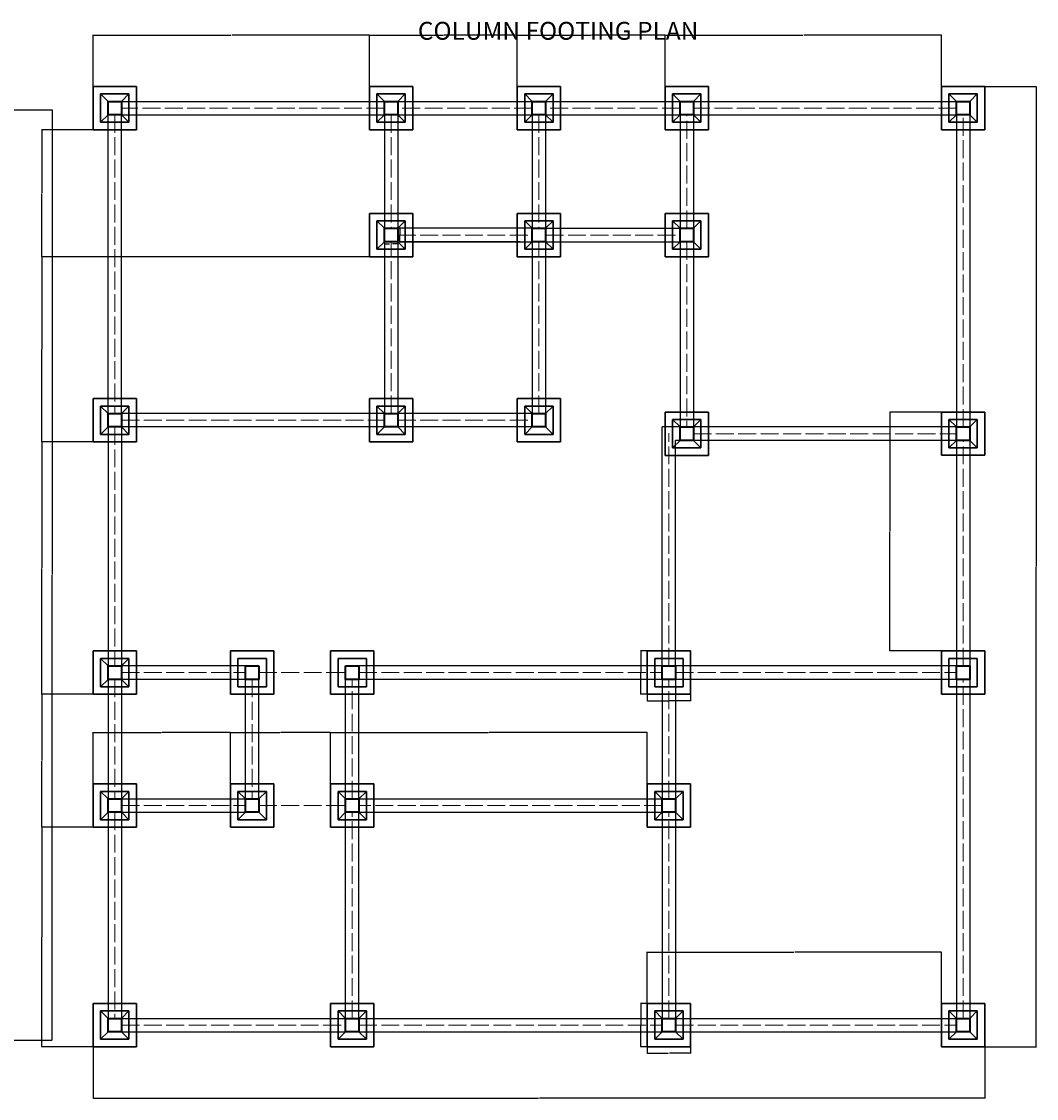
# Model space of a CAD drawing. Units: inches. Extents: x -1138 to 192, y 31 to 760.
# Tile 6 of 6: x -488 to 192, y 39 to 760. Entities that reach past the tile are written whole.
import ezdxf

# ---------------------------------------------------------------- set-up
doc = ezdxf.new("R2010")
doc.units = ezdxf.units.IN
doc.header["$MEASUREMENT"] = 0
doc.linetypes.add('ACAD_ISO02W100', pattern=[15, 12, -3])
for name, color, linetype, lineweight in [('A-ANNO-DIMS', 2, 'Continuous', 18), ('S-ANNO-TEXT', 7, 'Continuous', 25), ('S-BEAM', 7, 'Continuous', 25), ('S-BEAM-CNTR', 3, 'ACAD_ISO02W100', 13), ('S-COLS', 1, 'Continuous', 35), ('S-FNDN', 7, 'Continuous', 30)]:
    doc.layers.add(name, color=color, linetype=linetype, lineweight=lineweight)
doc.styles.get("Standard").update_dxf_attribs({"font": 'arial.ttf'})
doc.dimstyles.get("Standard").update_dxf_attribs({"dimtxt": 0.18, "dimasz": 0.18, "dimexe": 0.18, "dimexo": 0.0625, "dimgap": 0.09, "dimtad": 0, "dimtih": 1, "dimtoh": 1, "dimdec": 1, "dimzin": 0, "dimdsep": 46, "dimlunit": 4, "dimtxsty": 'Standard', "dimcen": 0.09, "dimadec": 0, "dimazin": 0, "dimtfac": 1, "dimtdec": 1, "dimtofl": 0, "dimtmove": 0, "dimatfit": 3, "dimfxl": 1, "dimtolj": 1, "dimtzin": 0, "dimarcsym": 0})

# ---------------------------------------------------------------- blocks, each defined once
blk = doc.blocks.new('COL-SQUARE-9IN')
for p, q in [((0, 9), (9, 9)), ((0, 0), (0, 9)), ((9, 9), (9, 0)), ((9, 0), (0, 0))]:
    blk.add_line(p, q)
blk = doc.blocks.new('FTG-29IN-SLOPED')
for p, q in [((0, 0), (0, 29)), ((0, 29), (29, 29)), ((29, 29), (29, 0)), ((5, 5), (5, 24)), ((5, 24), (24, 24)), ((5, 24), (10, 19)), ((19, 19), (24, 24)), ((24, 24), (24, 5)), ((5, 5), (10, 10)), ((19, 10), (24, 5)), ((24, 5), (5, 5)), ((29, 0), (0, 0))]:
    blk.add_line(p, q)
blk = doc.blocks.new('FTG-29IN-STEPPED')
for p, q in [((0, 0), (0, 29)), ((0, 29), (29, 29)), ((29, 29), (29, 0)), ((5, 5), (5, 24)), ((5, 24), (24, 24)), ((24, 24), (24, 5)), ((24, 5), (5, 5)), ((29, 0), (0, 0))]:
    blk.add_line(p, q)
blk = doc.blocks.new('*D39')
at = {"layer": 'A-ANNO-DIMS', "color": 0, "lineweight": -2, "transparency": 16777216}
for p, q in [((-244.81, 612.31), (-244.81, 610.84)), ((-244.63, 611.02), (-241.35, 611.02)), ((-235.99, 611.02), (-239.27, 611.02)), ((-235.81, 612.31), (-235.81, 610.84))]:
    blk.add_line(p, q, dxfattribs=at)
at = {"layer": 'A-ANNO-DIMS', "color": 0, "transparency": 16777216}
for points in [[(-244.63, 611.05), (-244.63, 610.99), (-244.81, 611.02)], [(-235.99, 611.05), (-235.99, 610.99), (-235.81, 611.02)]]:
    blk.add_solid(points, dxfattribs=at)
at = {"layer": 'Defpoints', "color": 0, "transparency": 16777216}
for p in [(-244.81, 612.37), (-235.81, 612.37), (-235.81, 611.02)]:
    blk.add_point(p, dxfattribs=at)
at = {"layer": 'A-ANNO-DIMS', "color": 0, "transparency": 16777216, "insert": (-240.31, 611.02), "char_height": 0.18, "attachment_point": 5}
blk.add_mtext('\\A1;COLUMN 9 TYP.', dxfattribs=at)
blk = doc.blocks.new('*D40')
at = {"layer": 'A-ANNO-DIMS', "color": 0, "lineweight": -2, "transparency": 16777216}
for p, q in [((-235.75, 621.37), (-234.28, 621.37)), ((-234.46, 621.19), (-234.46, 617.05)), ((-234.46, 612.55), (-234.46, 616.69)), ((-235.75, 612.37), (-234.28, 612.37))]:
    blk.add_line(p, q, dxfattribs=at)
at = {"layer": 'A-ANNO-DIMS', "color": 0, "transparency": 16777216}
for points in [[(-234.49, 621.19), (-234.43, 621.19), (-234.46, 621.37)], [(-234.49, 612.55), (-234.43, 612.55), (-234.46, 612.37)]]:
    blk.add_solid(points, dxfattribs=at)
at = {"layer": 'Defpoints', "color": 0, "transparency": 16777216}
for p in [(-235.81, 621.37), (-234.46, 621.37), (-235.81, 612.37)]:
    blk.add_point(p, dxfattribs=at)
at = {"layer": 'A-ANNO-DIMS', "color": 0, "transparency": 16777216, "insert": (-234.46, 616.87), "char_height": 0.18, "attachment_point": 5}
blk.add_mtext('\\A1;9 TYP.', dxfattribs=at)
blk = doc.blocks.new('*D41')
at = {"layer": 'A-ANNO-DIMS', "color": 0, "lineweight": -2, "transparency": 16777216}
for p, q in [((-68.87, 102.37), (-73.34, 102.37)), ((-73.16, 102.19), (-73.16, 88.05)), ((-73.16, 73.55), (-73.16, 87.69)), ((-68.87, 73.37), (-73.34, 73.37))]:
    blk.add_line(p, q, dxfattribs=at)
at = {"layer": 'A-ANNO-DIMS', "color": 0, "transparency": 16777216}
for points in [[(-73.19, 102.19), (-73.13, 102.19), (-73.16, 102.37)], [(-73.19, 73.55), (-73.13, 73.55), (-73.16, 73.37)]]:
    blk.add_solid(points, dxfattribs=at)
at = {"layer": 'Defpoints', "color": 0, "transparency": 16777216}
for p in [(-68.81, 102.37), (-73.16, 73.37), (-68.81, 73.37)]:
    blk.add_point(p, dxfattribs=at)
at = {"layer": 'A-ANNO-DIMS', "color": 0, "transparency": 16777216, "insert": (-73.16, 87.87), "char_height": 0.18, "attachment_point": 5}
blk.add_mtext('\\A1;SLOPED FOOTING 29 TYP.', dxfattribs=at)
blk = doc.blocks.new('*D42')
at = {"layer": 'A-ANNO-DIMS', "color": 0, "lineweight": -2, "transparency": 16777216}
for p, q in [((-68.81, 73.31), (-68.81, 68.84)), ((-39.81, 73.31), (-39.81, 68.84)), ((-68.63, 69.02), (-54.84, 69.02)), ((-39.99, 69.02), (-53.78, 69.02))]:
    blk.add_line(p, q, dxfattribs=at)
at = {"layer": 'A-ANNO-DIMS', "color": 0, "transparency": 16777216}
for points in [[(-68.63, 69.05), (-68.63, 68.99), (-68.81, 69.02)], [(-39.99, 69.05), (-39.99, 68.99), (-39.81, 69.02)]]:
    blk.add_solid(points, dxfattribs=at)
at = {"layer": 'Defpoints', "color": 0, "transparency": 16777216}
for p in [(-68.81, 73.37), (-39.81, 73.37), (-39.81, 69.02)]:
    blk.add_point(p, dxfattribs=at)
at = {"layer": 'A-ANNO-DIMS', "color": 0, "transparency": 16777216, "insert": (-54.31, 69.02), "char_height": 0.18, "attachment_point": 5}
blk.add_mtext('\\A1;29 TYP.', dxfattribs=at)
blk = doc.blocks.new('*D43')
at = {"layer": 'A-ANNO-DIMS', "color": 0, "lineweight": -2, "transparency": 16777216}
for p, q in [((-68.87, 338.37), (-73.34, 338.37)), ((-73.16, 338.19), (-73.16, 324.05)), ((-73.16, 309.55), (-73.16, 323.69)), ((-68.87, 309.37), (-73.34, 309.37))]:
    blk.add_line(p, q, dxfattribs=at)
at = {"layer": 'A-ANNO-DIMS', "color": 0, "transparency": 16777216}
for points in [[(-73.19, 338.19), (-73.13, 338.19), (-73.16, 338.37)], [(-73.19, 309.55), (-73.13, 309.55), (-73.16, 309.37)]]:
    blk.add_solid(points, dxfattribs=at)
at = {"layer": 'Defpoints', "color": 0, "transparency": 16777216}
for p in [(-68.81, 338.37), (-73.16, 309.37), (-68.81, 309.37)]:
    blk.add_point(p, dxfattribs=at)
at = {"layer": 'A-ANNO-DIMS', "color": 0, "transparency": 16777216, "insert": (-73.16, 323.87), "char_height": 0.18, "attachment_point": 5}
blk.add_mtext('\\A1;STEPPED FOOTING 29 TYP.', dxfattribs=at)
blk = doc.blocks.new('*D44')
at = {"layer": 'A-ANNO-DIMS', "color": 0, "lineweight": -2, "transparency": 16777216}
for p, q in [((-68.81, 309.31), (-68.81, 304.84)), ((-68.63, 305.02), (-54.84, 305.02)), ((-39.99, 305.02), (-53.78, 305.02)), ((-39.81, 309.31), (-39.81, 304.84))]:
    blk.add_line(p, q, dxfattribs=at)
at = {"layer": 'A-ANNO-DIMS', "color": 0, "transparency": 16777216}
for points in [[(-68.63, 305.05), (-68.63, 304.99), (-68.81, 305.02)], [(-39.99, 305.05), (-39.99, 304.99), (-39.81, 305.02)]]:
    blk.add_solid(points, dxfattribs=at)
at = {"layer": 'Defpoints', "color": 0, "transparency": 16777216}
for p in [(-68.81, 309.37), (-39.81, 309.37), (-39.81, 305.02)]:
    blk.add_point(p, dxfattribs=at)
at = {"layer": 'A-ANNO-DIMS', "color": 0, "transparency": 16777216, "insert": (-54.31, 305.02), "char_height": 0.18, "attachment_point": 5}
blk.add_mtext('\\A1;29 TYP.', dxfattribs=at)
blk = doc.blocks.new('*D86')
at = {"layer": 'A-ANNO-DIMS', "color": 0, "lineweight": -2, "transparency": 16777216}
for p, q in [((-514.07, 700.81), (-467.14, 700.81)), ((-467.32, 700.63), (-467.32, 389.49)), ((-467.32, 77.99), (-467.32, 389.13)), ((-514.07, 77.81), (-467.14, 77.81))]:
    blk.add_line(p, q, dxfattribs=at)
at = {"layer": 'A-ANNO-DIMS', "color": 0, "transparency": 16777216}
for points in [[(-467.35, 700.63), (-467.29, 700.63), (-467.32, 700.81)], [(-467.35, 77.99), (-467.29, 77.99), (-467.32, 77.81)]]:
    blk.add_solid(points, dxfattribs=at)
at = {"layer": 'Defpoints', "color": 0, "transparency": 16777216}
for p in [(-514.13, 700.81), (-467.32, 700.81), (-514.13, 77.81)]:
    blk.add_point(p, dxfattribs=at)
at = {"layer": 'A-ANNO-DIMS', "color": 0, "transparency": 16777216, "insert": (-467.32, 389.31), "char_height": 0.18, "attachment_point": 5}
blk.add_mtext('\\A1;623', dxfattribs=at)
blk = doc.blocks.new('*D105')
at = {"layer": 'A-ANNO-DIMS', "color": 0, "lineweight": -2, "transparency": 16777216}
for p, q in [((-439.81, 73.31), (-439.81, 38.76)), ((157.19, 73.31), (157.19, 38.76)), ((-439.63, 38.94), (-141.6, 38.94)), ((157.01, 38.94), (-141.02, 38.94))]:
    blk.add_line(p, q, dxfattribs=at)
at = {"layer": 'A-ANNO-DIMS', "color": 0, "transparency": 16777216}
for points in [[(-439.63, 38.97), (-439.63, 38.91), (-439.81, 38.94)], [(157.01, 38.97), (157.01, 38.91), (157.19, 38.94)]]:
    blk.add_solid(points, dxfattribs=at)
at = {"layer": 'Defpoints', "color": 0, "transparency": 16777216}
for p in [(-439.81, 73.37), (157.19, 73.37), (157.19, 38.94)]:
    blk.add_point(p, dxfattribs=at)
at = {"layer": 'A-ANNO-DIMS', "color": 0, "transparency": 16777216, "insert": (-141.31, 38.94), "char_height": 0.18, "attachment_point": 5}
blk.add_mtext('\\A1;597', dxfattribs=at)
blk = doc.blocks.new('*D106')
at = {"layer": 'A-ANNO-DIMS', "color": 0, "lineweight": -2, "transparency": 16777216}
for p, q in [((157.25, 716.37), (191.81, 716.37)), ((191.63, 716.19), (191.63, 395.05)), ((191.63, 73.55), (191.63, 394.69)), ((157.25, 73.37), (191.81, 73.37))]:
    blk.add_line(p, q, dxfattribs=at)
at = {"layer": 'A-ANNO-DIMS', "color": 0, "transparency": 16777216}
for points in [[(191.6, 716.19), (191.66, 716.19), (191.63, 716.37)], [(191.6, 73.55), (191.66, 73.55), (191.63, 73.37)]]:
    blk.add_solid(points, dxfattribs=at)
at = {"layer": 'Defpoints', "color": 0, "transparency": 16777216}
for p in [(157.19, 716.37), (191.63, 716.37), (157.19, 73.37)]:
    blk.add_point(p, dxfattribs=at)
at = {"layer": 'A-ANNO-DIMS', "color": 0, "transparency": 16777216, "insert": (191.63, 394.87), "char_height": 0.18, "attachment_point": 5}
blk.add_mtext('\\A1;643', dxfattribs=at)
blk = doc.blocks.new('*D107')
at = {"layer": 'A-ANNO-DIMS', "color": 0, "lineweight": -2, "transparency": 16777216}
for p, q in [((-439.81, 716.43), (-439.81, 750.99)), ((-439.63, 750.81), (-347.59, 750.81)), ((-254.99, 750.81), (-347.03, 750.81)), ((-254.81, 716.43), (-254.81, 750.99))]:
    blk.add_line(p, q, dxfattribs=at)
at = {"layer": 'A-ANNO-DIMS', "color": 0, "transparency": 16777216}
for points in [[(-439.63, 750.84), (-439.63, 750.78), (-439.81, 750.81)], [(-254.99, 750.84), (-254.99, 750.78), (-254.81, 750.81)]]:
    blk.add_solid(points, dxfattribs=at)
at = {"layer": 'Defpoints', "color": 0, "transparency": 16777216}
for p in [(-254.81, 750.81), (-439.81, 716.37), (-254.81, 716.37)]:
    blk.add_point(p, dxfattribs=at)
at = {"layer": 'A-ANNO-DIMS', "color": 0, "transparency": 16777216, "insert": (-347.31, 750.81), "char_height": 0.18, "attachment_point": 5}
blk.add_mtext('\\A1;185', dxfattribs=at)
blk = doc.blocks.new('*D108')
at = {"layer": 'A-ANNO-DIMS', "color": 0, "lineweight": -2, "transparency": 16777216}
for p, q in [((-254.81, 716.43), (-254.81, 750.99)), ((-254.63, 750.81), (-205.53, 750.81)), ((-155.99, 750.81), (-205.09, 750.81)), ((-155.81, 716.43), (-155.81, 750.99))]:
    blk.add_line(p, q, dxfattribs=at)
at = {"layer": 'A-ANNO-DIMS', "color": 0, "transparency": 16777216}
for points in [[(-254.63, 750.84), (-254.63, 750.78), (-254.81, 750.81)], [(-155.99, 750.84), (-155.99, 750.78), (-155.81, 750.81)]]:
    blk.add_solid(points, dxfattribs=at)
at = {"layer": 'Defpoints', "color": 0, "transparency": 16777216}
for p in [(-155.81, 750.81), (-254.81, 716.37), (-155.81, 716.37)]:
    blk.add_point(p, dxfattribs=at)
at = {"layer": 'A-ANNO-DIMS', "color": 0, "transparency": 16777216, "insert": (-205.31, 750.81), "char_height": 0.18, "attachment_point": 5}
blk.add_mtext('\\A1;99', dxfattribs=at)
blk = doc.blocks.new('*D109')
at = {"layer": 'A-ANNO-DIMS', "color": 0, "lineweight": -2, "transparency": 16777216}
for p, q in [((-155.81, 716.43), (-155.81, 750.99)), ((-155.63, 750.81), (-106.53, 750.81)), ((-56.99, 750.81), (-106.09, 750.81)), ((-56.81, 716.43), (-56.81, 750.99))]:
    blk.add_line(p, q, dxfattribs=at)
at = {"layer": 'A-ANNO-DIMS', "color": 0, "transparency": 16777216}
for points in [[(-155.63, 750.84), (-155.63, 750.78), (-155.81, 750.81)], [(-56.99, 750.84), (-56.99, 750.78), (-56.81, 750.81)]]:
    blk.add_solid(points, dxfattribs=at)
at = {"layer": 'Defpoints', "color": 0, "transparency": 16777216}
for p in [(-56.81, 750.81), (-155.81, 716.37), (-56.81, 716.37)]:
    blk.add_point(p, dxfattribs=at)
at = {"layer": 'A-ANNO-DIMS', "color": 0, "transparency": 16777216, "insert": (-106.31, 750.81), "char_height": 0.18, "attachment_point": 5}
blk.add_mtext('\\A1;99', dxfattribs=at)
blk = doc.blocks.new('*D110')
at = {"layer": 'A-ANNO-DIMS', "color": 0, "lineweight": -2, "transparency": 16777216}
for p, q in [((-56.81, 716.43), (-56.81, 750.99)), ((-56.63, 750.81), (35.41, 750.81)), ((128.01, 750.81), (35.97, 750.81)), ((128.19, 716.43), (128.19, 750.99))]:
    blk.add_line(p, q, dxfattribs=at)
at = {"layer": 'A-ANNO-DIMS', "color": 0, "transparency": 16777216}
for points in [[(-56.63, 750.84), (-56.63, 750.78), (-56.81, 750.81)], [(128.01, 750.84), (128.01, 750.78), (128.19, 750.81)]]:
    blk.add_solid(points, dxfattribs=at)
at = {"layer": 'Defpoints', "color": 0, "transparency": 16777216}
for p in [(128.19, 750.81), (-56.81, 716.37), (128.19, 716.37)]:
    blk.add_point(p, dxfattribs=at)
at = {"layer": 'A-ANNO-DIMS', "color": 0, "transparency": 16777216, "insert": (35.69, 750.81), "char_height": 0.18, "attachment_point": 5}
blk.add_mtext('\\A1;185', dxfattribs=at)
blk = doc.blocks.new('*D111')
at = {"layer": 'A-ANNO-DIMS', "color": 0, "lineweight": -2, "transparency": 16777216}
for p, q in [((-439.87, 220.37), (-474.42, 220.37)), ((-474.24, 220.19), (-474.24, 147.05)), ((-474.24, 73.55), (-474.24, 146.69)), ((-439.87, 73.37), (-474.42, 73.37))]:
    blk.add_line(p, q, dxfattribs=at)
at = {"layer": 'A-ANNO-DIMS', "color": 0, "transparency": 16777216}
for points in [[(-474.27, 220.19), (-474.21, 220.19), (-474.24, 220.37)], [(-474.27, 73.55), (-474.21, 73.55), (-474.24, 73.37)]]:
    blk.add_solid(points, dxfattribs=at)
at = {"layer": 'Defpoints', "color": 0, "transparency": 16777216}
for p in [(-474.24, 220.37), (-439.81, 220.37), (-439.81, 73.37)]:
    blk.add_point(p, dxfattribs=at)
at = {"layer": 'A-ANNO-DIMS', "color": 0, "transparency": 16777216, "insert": (-474.24, 146.87), "char_height": 0.18, "attachment_point": 5}
blk.add_mtext('\\A1;147', dxfattribs=at)
blk = doc.blocks.new('*D112')
at = {"layer": 'A-ANNO-DIMS', "color": 0, "lineweight": -2, "transparency": 16777216}
for p, q in [((-439.87, 309.37), (-474.42, 309.37)), ((-474.24, 309.19), (-474.24, 265.05)), ((-474.24, 220.55), (-474.24, 264.69)), ((-439.87, 220.37), (-474.42, 220.37))]:
    blk.add_line(p, q, dxfattribs=at)
at = {"layer": 'A-ANNO-DIMS', "color": 0, "transparency": 16777216}
for points in [[(-474.27, 309.19), (-474.21, 309.19), (-474.24, 309.37)], [(-474.27, 220.55), (-474.21, 220.55), (-474.24, 220.37)]]:
    blk.add_solid(points, dxfattribs=at)
at = {"layer": 'Defpoints', "color": 0, "transparency": 16777216}
for p in [(-474.24, 309.37), (-439.81, 309.37), (-439.81, 220.37)]:
    blk.add_point(p, dxfattribs=at)
at = {"layer": 'A-ANNO-DIMS', "color": 0, "transparency": 16777216, "insert": (-474.24, 264.87), "char_height": 0.18, "attachment_point": 5}
blk.add_mtext('\\A1;89', dxfattribs=at)
blk = doc.blocks.new('*D113')
at = {"layer": 'A-ANNO-DIMS', "color": 0, "lineweight": -2, "transparency": 16777216}
for p, q in [((-439.87, 478.37), (-474.42, 478.37)), ((-474.24, 478.19), (-474.24, 394.05)), ((-474.24, 309.55), (-474.24, 393.69)), ((-439.87, 309.37), (-474.42, 309.37))]:
    blk.add_line(p, q, dxfattribs=at)
at = {"layer": 'A-ANNO-DIMS', "color": 0, "transparency": 16777216}
for points in [[(-474.27, 478.19), (-474.21, 478.19), (-474.24, 478.37)], [(-474.27, 309.55), (-474.21, 309.55), (-474.24, 309.37)]]:
    blk.add_solid(points, dxfattribs=at)
at = {"layer": 'Defpoints', "color": 0, "transparency": 16777216}
for p in [(-474.24, 478.37), (-439.81, 478.37), (-439.81, 309.37)]:
    blk.add_point(p, dxfattribs=at)
at = {"layer": 'A-ANNO-DIMS', "color": 0, "transparency": 16777216, "insert": (-474.24, 393.87), "char_height": 0.18, "attachment_point": 5}
blk.add_mtext('\\A1;169', dxfattribs=at)
blk = doc.blocks.new('*D114')
at = {"layer": 'A-ANNO-DIMS', "color": 0, "lineweight": -2, "transparency": 16777216}
for p, q in [((-254.87, 602.37), (-474.42, 602.37)), ((-474.24, 602.19), (-474.24, 540.55)), ((-474.24, 478.55), (-474.24, 540.19)), ((-439.87, 478.37), (-474.42, 478.37))]:
    blk.add_line(p, q, dxfattribs=at)
at = {"layer": 'A-ANNO-DIMS', "color": 0, "transparency": 16777216}
for points in [[(-474.27, 602.19), (-474.21, 602.19), (-474.24, 602.37)], [(-474.27, 478.55), (-474.21, 478.55), (-474.24, 478.37)]]:
    blk.add_solid(points, dxfattribs=at)
at = {"layer": 'Defpoints', "color": 0, "transparency": 16777216}
for p in [(-474.24, 602.37), (-254.81, 602.37), (-439.81, 478.37)]:
    blk.add_point(p, dxfattribs=at)
at = {"layer": 'A-ANNO-DIMS', "color": 0, "transparency": 16777216, "insert": (-474.24, 540.37), "char_height": 0.18, "attachment_point": 5}
blk.add_mtext('\\A1;124', dxfattribs=at)
blk = doc.blocks.new('*D115')
at = {"layer": 'A-ANNO-DIMS', "color": 0, "lineweight": -2, "transparency": 16777216}
for p, q in [((-439.87, 687.37), (-474.42, 687.37)), ((-474.24, 687.19), (-474.24, 645.05)), ((-474.24, 602.55), (-474.24, 644.69)), ((-254.87, 602.37), (-474.42, 602.37))]:
    blk.add_line(p, q, dxfattribs=at)
at = {"layer": 'A-ANNO-DIMS', "color": 0, "transparency": 16777216}
for points in [[(-474.27, 687.19), (-474.21, 687.19), (-474.24, 687.37)], [(-474.27, 602.55), (-474.21, 602.55), (-474.24, 602.37)]]:
    blk.add_solid(points, dxfattribs=at)
at = {"layer": 'Defpoints', "color": 0, "transparency": 16777216}
for p in [(-474.24, 687.37), (-439.81, 687.37), (-254.81, 602.37)]:
    blk.add_point(p, dxfattribs=at)
at = {"layer": 'A-ANNO-DIMS', "color": 0, "transparency": 16777216, "insert": (-474.24, 644.87), "char_height": 0.18, "attachment_point": 5}
blk.add_mtext('\\A1;85', dxfattribs=at)
blk = doc.blocks.new('*D116')
at = {"layer": 'A-ANNO-DIMS', "color": 0, "lineweight": -2, "transparency": 16777216}
for p, q in [((-439.81, 249.43), (-439.81, 283.99)), ((-439.63, 283.81), (-394.03, 283.81)), ((-347.99, 283.81), (-393.59, 283.81)), ((-347.81, 249.43), (-347.81, 283.99))]:
    blk.add_line(p, q, dxfattribs=at)
at = {"layer": 'A-ANNO-DIMS', "color": 0, "transparency": 16777216}
for points in [[(-439.63, 283.84), (-439.63, 283.78), (-439.81, 283.81)], [(-347.99, 283.84), (-347.99, 283.78), (-347.81, 283.81)]]:
    blk.add_solid(points, dxfattribs=at)
at = {"layer": 'Defpoints', "color": 0, "transparency": 16777216}
for p in [(-347.81, 283.81), (-439.81, 249.37), (-347.81, 249.37)]:
    blk.add_point(p, dxfattribs=at)
at = {"layer": 'A-ANNO-DIMS', "color": 0, "transparency": 16777216, "insert": (-393.81, 283.81), "char_height": 0.18, "attachment_point": 5}
blk.add_mtext('\\A1;92', dxfattribs=at)
blk = doc.blocks.new('*D117')
at = {"layer": 'A-ANNO-DIMS', "color": 0, "lineweight": -2, "transparency": 16777216}
for p, q in [((-347.81, 249.43), (-347.81, 283.99)), ((-347.63, 283.81), (-314.53, 283.81)), ((-280.99, 283.81), (-314.09, 283.81)), ((-280.81, 249.43), (-280.81, 283.99))]:
    blk.add_line(p, q, dxfattribs=at)
at = {"layer": 'A-ANNO-DIMS', "color": 0, "transparency": 16777216}
for points in [[(-347.63, 283.84), (-347.63, 283.78), (-347.81, 283.81)], [(-280.99, 283.84), (-280.99, 283.78), (-280.81, 283.81)]]:
    blk.add_solid(points, dxfattribs=at)
at = {"layer": 'Defpoints', "color": 0, "transparency": 16777216}
for p in [(-280.81, 283.81), (-347.81, 249.37), (-280.81, 249.37)]:
    blk.add_point(p, dxfattribs=at)
at = {"layer": 'A-ANNO-DIMS', "color": 0, "transparency": 16777216, "insert": (-314.31, 283.81), "char_height": 0.18, "attachment_point": 5}
blk.add_mtext('\\A1;67', dxfattribs=at)
blk = doc.blocks.new('*D118')
at = {"layer": 'A-ANNO-DIMS', "color": 0, "lineweight": -2, "transparency": 16777216}
for p, q in [((-280.81, 249.43), (-280.81, 283.99)), ((-280.63, 283.81), (-175.1, 283.81)), ((-68.99, 283.81), (-174.52, 283.81)), ((-68.81, 249.43), (-68.81, 283.99))]:
    blk.add_line(p, q, dxfattribs=at)
at = {"layer": 'A-ANNO-DIMS', "color": 0, "transparency": 16777216}
for points in [[(-280.63, 283.84), (-280.63, 283.78), (-280.81, 283.81)], [(-68.99, 283.84), (-68.99, 283.78), (-68.81, 283.81)]]:
    blk.add_solid(points, dxfattribs=at)
at = {"layer": 'Defpoints', "color": 0, "transparency": 16777216}
for p in [(-68.81, 283.81), (-280.81, 249.37), (-68.81, 249.37)]:
    blk.add_point(p, dxfattribs=at)
at = {"layer": 'A-ANNO-DIMS', "color": 0, "transparency": 16777216, "insert": (-174.81, 283.81), "char_height": 0.18, "attachment_point": 5}
blk.add_mtext('\\A1;212', dxfattribs=at)
blk = doc.blocks.new('*D119')
at = {"layer": 'A-ANNO-DIMS', "color": 0, "lineweight": -2, "transparency": 16777216}
for p, q in [((-68.81, 102.43), (-68.81, 136.99)), ((-68.63, 136.81), (29.41, 136.81)), ((128.01, 136.81), (29.97, 136.81)), ((128.19, 102.43), (128.19, 136.99))]:
    blk.add_line(p, q, dxfattribs=at)
at = {"layer": 'A-ANNO-DIMS', "color": 0, "transparency": 16777216}
for points in [[(-68.63, 136.84), (-68.63, 136.78), (-68.81, 136.81)], [(128.01, 136.84), (128.01, 136.78), (128.19, 136.81)]]:
    blk.add_solid(points, dxfattribs=at)
at = {"layer": 'Defpoints', "color": 0, "transparency": 16777216}
for p in [(128.19, 136.81), (-68.81, 102.37), (128.19, 102.37)]:
    blk.add_point(p, dxfattribs=at)
at = {"layer": 'A-ANNO-DIMS', "color": 0, "transparency": 16777216, "insert": (29.69, 136.81), "char_height": 0.18, "attachment_point": 5}
blk.add_mtext('\\A1;197', dxfattribs=at)
blk = doc.blocks.new('*D120')
at = {"layer": 'A-ANNO-DIMS', "color": 0, "lineweight": -2, "transparency": 16777216}
for p, q in [((128.13, 498.37), (93.58, 498.37)), ((93.76, 498.19), (93.76, 418.55)), ((93.76, 338.55), (93.76, 418.19)), ((128.13, 338.37), (93.58, 338.37))]:
    blk.add_line(p, q, dxfattribs=at)
at = {"layer": 'A-ANNO-DIMS', "color": 0, "transparency": 16777216}
for points in [[(93.73, 498.19), (93.79, 498.19), (93.76, 498.37)], [(93.73, 338.55), (93.79, 338.55), (93.76, 338.37)]]:
    blk.add_solid(points, dxfattribs=at)
at = {"layer": 'Defpoints', "color": 0, "transparency": 16777216}
for p in [(93.76, 498.37), (128.19, 498.37), (128.19, 338.37)]:
    blk.add_point(p, dxfattribs=at)
at = {"layer": 'A-ANNO-DIMS', "color": 0, "transparency": 16777216, "insert": (93.76, 418.37), "char_height": 0.18, "attachment_point": 5}
blk.add_mtext('\\A1;160', dxfattribs=at)

msp = doc.modelspace()

# ---------------------------------------------------------------- linework, layer by layer
at = {"layer": 'S-BEAM'}
for p, q in [((-429.808, 706.372), (-235.808, 706.372)), ((-429.808, 497.372), (-429.808, 706.372)), ((-235.808, 706.372), (-136.808, 706.372)), ((-136.808, 706.372), (-37.808, 706.372)), ((-37.808, 706.372), (147.192, 706.372)), ((147.192, 706.372), (147.192, 488.372)), ((-420.808, 697.372), (-244.808, 697.372)), ((-420.808, 497.372), (-420.808, 697.372)), ((-244.808, 697.372), (-244.808, 616.872)), ((-235.808, 697.372), (-235.808, 621.372)), ((-235.808, 697.372), (-145.808, 697.372)), ((-145.808, 697.372), (-145.808, 621.372)), ((-136.808, 697.372), (-136.808, 621.372)), ((-136.808, 697.372), (-46.808, 697.372)), ((-46.808, 697.372), (-46.808, 650.462)), ((-46.808, 697.372), (-46.808, 621.372)), ((-37.808, 697.372), (-37.808, 621.372)), ((-37.808, 697.372), (138.192, 697.372)), ((138.192, 697.372), (138.192, 488.372)), ((-145.808, 621.372), (-235.808, 621.372)), ((-136.808, 621.372), (-46.808, 621.372)), ((-37.808, 621.372), (-37.808, 488.372)), ((-244.808, 616.872), (-244.808, 497.372)), ((-235.808, 612.372), (-235.808, 497.372)), ((-153.808, 612.372), (-235.808, 612.372)), ((-235.808, 612.372), (-145.808, 612.372)), ((-145.808, 612.372), (-145.808, 497.372)), ((-136.808, 612.372), (-136.808, 488.372)), ((-136.808, 612.372), (-46.808, 612.372)), ((-46.808, 612.372), (-46.808, 488.372)), ((-429.808, 497.372), (-429.808, 300.372)), ((-284.696, 497.372), (-420.808, 497.372)), ((-244.808, 497.372), (-420.808, 497.372)), ((-145.808, 497.372), (-235.808, 497.372)), ((-244.808, 488.372), (-420.808, 488.372)), ((-420.808, 488.372), (-420.808, 328.372)), ((-136.808, 488.372), (-244.808, 488.372)), ((-58.808, 328.372), (-58.808, 488.372)), ((-46.808, 488.372), (-58.808, 488.372)), ((138.192, 488.372), (-37.808, 488.372)), ((138.192, 488.372), (-37.808, 488.372)), ((147.192, 488.372), (147.192, 328.372)), ((138.192, 479.372), (-49.808, 479.372)), ((-49.808, 328.372), (-49.808, 479.372)), ((138.192, 479.372), (138.192, 328.372)), ((138.192, 377.372), (138.192, 328.372)), ((147.192, 377.372), (147.192, 83.372)), ((-328.808, 328.372), (-420.808, 328.372)), ((-328.808, 230.372), (-328.808, 328.372)), ((-58.808, 328.372), (-270.808, 328.372)), ((-270.808, 92.372), (-270.808, 328.372)), ((138.192, 328.372), (-49.808, 328.372)), ((-429.808, 319.372), (-429.808, 239.372)), ((-337.808, 319.372), (-420.808, 319.372)), ((-420.808, 319.372), (-420.808, 239.372)), ((-337.808, 239.372), (-337.808, 319.372)), ((-58.808, 319.372), (-261.808, 319.372)), ((-261.808, 239.372), (-261.808, 319.372)), ((-58.808, 319.372), (-58.808, 239.372)), ((138.192, 319.372), (-49.808, 319.372)), ((-49.808, 319.372), (-49.808, 230.372)), ((138.192, 319.372), (138.192, 92.372)), ((-429.808, 239.372), (-429.808, 83.372)), ((-420.808, 239.372), (-337.808, 239.372)), ((-391.718, 239.372), (-337.808, 239.372)), ((-261.808, 239.372), (-58.808, 239.372)), ((-420.808, 230.372), (-420.808, 92.372)), ((-420.808, 230.372), (-328.808, 230.372)), ((-261.808, 92.372), (-261.808, 230.372)), ((-261.808, 230.372), (-49.808, 230.372)), ((-58.808, 230.372), (-58.808, 92.372)), ((-49.808, 230.372), (-49.808, 92.372)), ((-420.808, 92.372), (-270.808, 92.372)), ((-261.808, 92.372), (138.192, 92.372)), ((-429.808, 83.372), (147.192, 83.372))]:
    msp.add_line(p, q, dxfattribs=at)
at = {"layer": 'S-BEAM-CNTR'}
for p, q in [((-244.808, 701.872), (-420.808, 701.872)), ((-145.808, 701.872), (-235.808, 701.872)), ((-46.808, 701.872), (-136.808, 701.872)), ((138.192, 701.872), (-37.808, 701.872)), ((-425.308, 697.372), (-425.308, 497.372)), ((-240.308, 697.372), (-240.308, 621.372)), ((-141.308, 697.372), (-141.308, 621.372)), ((-42.308, 621.372), (-42.308, 697.372)), ((142.692, 488.372), (142.692, 697.372)), ((-235.808, 616.872), (-145.808, 616.872)), ((-136.808, 616.872), (-46.808, 616.872)), ((-240.308, 497.372), (-240.308, 612.372)), ((-141.308, 497.372), (-141.308, 612.372)), ((-42.308, 612.372), (-42.308, 488.372)), ((-420.808, 492.872), (-244.808, 492.872)), ((-235.808, 492.872), (-145.808, 492.872)), ((-425.308, 488.372), (-425.308, 328.372)), ((-54.308, 328.372), (-54.308, 484.165)), ((-37.808, 483.872), (138.192, 483.872)), ((142.692, 328.372), (142.692, 479.372)), ((-425.308, 319.372), (-425.308, 239.372)), ((-420.808, 323.872), (-337.808, 323.872)), ((-333.308, 319.372), (-333.308, 239.372)), ((-328.808, 323.872), (-270.808, 323.872)), ((-266.308, 239.372), (-266.308, 319.372)), ((-261.808, 323.872), (-58.808, 323.872)), ((-54.308, 239.372), (-54.308, 319.372)), ((-49.808, 323.872), (138.192, 323.872)), ((142.692, 92.372), (142.692, 319.372)), ((-420.808, 234.872), (-337.808, 234.872)), ((-328.808, 234.872), (-270.808, 234.872)), ((-58.808, 234.872), (-261.808, 234.872)), ((-425.308, 230.372), (-425.308, 92.372)), ((-266.308, 92.372), (-266.308, 230.372)), ((-54.308, 92.372), (-54.308, 230.372)), ((-420.808, 87.872), (-270.808, 87.872)), ((-261.808, 87.872), (-58.808, 87.872)), ((-49.808, 87.872), (138.192, 87.872))]:
    msp.add_line(p, q, dxfattribs=at)

# ---------------------------------------------------------------- block references
at = {"layer": 'S-COLS'}
for p in [(-429.808, 697.372), (-244.808, 697.372), (-145.808, 697.372), (-46.808, 697.372), (138.192, 697.372), (-244.808, 612.372), (-145.808, 612.372), (-46.808, 612.372), (-429.808, 488.372), (-244.808, 488.372), (-145.808, 488.372), (-46.808, 479.372), (138.192, 479.372), (-429.808, 319.372), (-337.808, 319.372), (-270.808, 319.372), (-58.808, 319.372), (138.192, 319.372), (-429.808, 230.372), (-337.808, 230.372), (-270.808, 230.372), (-58.808, 230.372), (-429.808, 83.372), (-270.808, 83.372), (-58.808, 83.372), (138.192, 83.372)]:
    msp.add_blockref('COL-SQUARE-9IN', p, dxfattribs=at)
at = {"layer": 'S-FNDN'}
for name, p, rotation in [('FTG-29IN-SLOPED', (-410.809, 687.372), 89.99999999999974), ('FTG-29IN-SLOPED', (-254.808, 716.371), 270.0000000000005), ('FTG-29IN-SLOPED', (-126.809, 687.372), 89.99999999999999), ('FTG-29IN-SLOPED', (-56.808, 716.371), 270.0000000000003), ('FTG-29IN-SLOPED', (157.191, 687.372), 89.99999999999984), ('FTG-29IN-SLOPED', (-225.808, 631.371), 180), ('FTG-29IN-SLOPED', (-155.808, 631.371), 270.0000000000005), ('FTG-29IN-SLOPED', (-439.808, 507.371), 270.0000000000004), ('FTG-29IN-SLOPED', (-254.808, 507.371), 269.9999999999998), ('FTG-29IN-SLOPED', (-155.808, 507.371), 270.0000000000003), ('FTG-29IN-SLOPED', (-56.808, 498.371), 270.0000000000002), ('FTG-29IN-SLOPED', (-410.808, 338.371), 180), ('FTG-29IN-STEPPED', (-251.809, 309.372), 89.99999999999979), ('FTG-29IN-STEPPED', (-68.808, 338.371), 270), ('FTG-29IN-SLOPED', (-439.808, 249.371), 270), ('FTG-29IN-SLOPED', (-347.808, 249.371), 269.9999999999995), ('FTG-29IN-SLOPED', (-280.808, 249.371), 270), ('FTG-29IN-SLOPED', (-280.808, 102.371), 270), ('FTG-29IN-SLOPED', (-68.808, 102.371), 270.0000000000001), ('FTG-29IN-SLOPED', (128.192, 102.371), 270.0000000000001)]:
    msp.add_blockref(name, p, dxfattribs=dict(at, rotation=rotation))
for name, p in [('FTG-29IN-SLOPED', (-56.808, 602.372)), ('FTG-29IN-SLOPED', (128.192, 469.372)), ('FTG-29IN-STEPPED', (-347.808, 309.372)), ('FTG-29IN-STEPPED', (128.192, 309.372)), ('FTG-29IN-SLOPED', (-68.808, 220.372)), ('FTG-29IN-SLOPED', (-439.808, 73.372))]:
    msp.add_blockref(name, p, dxfattribs=at)

# ---------------------------------------------------------------- texts
at = {"layer": 'S-ANNO-TEXT'}
msp.add_text('COLUMN FOOTING PLAN', height=12, dxfattribs=at).set_placement((-222.383, 747.611))

# ---------------------------------------------------------------- dimensions: what is measured, and where the dimension line sits
at = {"layer": 'A-ANNO-DIMS'}
for base, p1, p2, picture, middle in [((-254.808, 750.807), (-439.808, 716.372), (-254.808, 716.372), '*D107', (-347.308, 750.807)), ((-155.808, 750.807), (-254.808, 716.372), (-155.808, 716.372), '*D108', (-205.308, 750.807)), ((-56.808, 750.807), (-155.808, 716.372), (-56.808, 716.372), '*D109', (-106.308, 750.807)), ((128.192, 750.807), (-56.808, 716.372), (128.192, 716.372), '*D110', (35.692, 750.807)), ((-280.808, 283.807), (-347.808, 249.372), (-280.808, 249.372), '*D117', (-314.308, 283.807)), ((-68.808, 283.807), (-280.808, 249.372), (-68.808, 249.372), '*D118', (-174.808, 283.807)), ((128.192, 136.807), (-68.808, 102.372), (128.192, 102.372), '*D119', (29.692, 136.807)), ((157.192, 38.937), (-439.808, 73.372), (157.192, 73.372), '*D105', (-141.308, 38.937))]:
    dim = msp.add_linear_dim(base=base, p1=p1, p2=p2, dimstyle='Standard', override={"dimdec": 0, "dimlfac": 1, "dimrnd": 0, "dimzin": 0, "dimdsep": 46, "dimlunit": 2}, dxfattribs=at)
    dim.commit()
    dim.dimension.update_dxf_attribs({"geometry": picture, "text_midpoint": middle})
for base, p1, p2, angle, picture, middle in [((191.627, 716.372), (157.192, 73.372), (157.192, 716.372), 90, '*D106', (191.627, 394.872)), ((-467.318, 700.813), (-514.133, 77.813), (-514.133, 700.813), 90, '*D86', (-467.318, 389.313)), ((-474.243, 687.372), (-254.808, 602.372), (-439.808, 687.372), 90, '*D115', (-474.243, 644.872)), ((-474.243, 602.372), (-439.808, 478.372), (-254.808, 602.372), 90, '*D114', (-474.243, 540.372)), ((93.757, 498.372), (128.192, 338.372), (128.192, 498.372), 90, '*D120', (93.757, 418.372)), ((-474.243, 478.372), (-439.808, 309.372), (-439.808, 478.372), 90, '*D113', (-474.243, 393.872)), ((-474.243, 309.372), (-439.808, 220.372), (-439.808, 309.372), 90, '*D112', (-474.243, 264.872)), ((-347.808, 283.807), (-439.808, 249.372), (-347.808, 249.372), 0, '*D116', (-393.808, 283.807)), ((-474.243, 220.372), (-439.808, 73.372), (-439.808, 220.372), 90, '*D111', (-474.243, 146.872))]:
    dim = msp.add_linear_dim(base=base, p1=p1, p2=p2, angle=angle, dimstyle='Standard', override={"dimdec": 0, "dimlfac": 1, "dimrnd": 0, "dimzin": 0, "dimdsep": 46, "dimlunit": 2}, dxfattribs=at)
    dim.commit()
    dim.dimension.update_dxf_attribs({"geometry": picture, "text_midpoint": middle})
for base, p1, p2, angle, text, picture, middle in [((-234.458, 621.372), (-235.808, 612.372), (-235.808, 621.372), 90, '<> TYP.', '*D40', (-234.458, 616.872)), ((-73.158, 309.372), (-68.808, 338.372), (-68.808, 309.372), 270, 'STEPPED FOOTING <> TYP.', '*D43', (-73.158, 323.872)), ((-73.158, 73.372), (-68.808, 102.372), (-68.808, 73.372), 270, 'SLOPED FOOTING <> TYP.', '*D41', (-73.158, 87.872)), ((-39.808, 69.022), (-68.808, 73.372), (-39.808, 73.372), 0, '<> TYP.', '*D42', (-54.308, 69.022))]:
    dim = msp.add_linear_dim(base=base, p1=p1, p2=p2, angle=angle, text=text, dimstyle='Standard', override={"dimdec": 0, "dimlfac": 1, "dimrnd": 0, "dimzin": 0, "dimdsep": 46, "dimlunit": 2}, dxfattribs=at)
    dim.commit()
    dim.dimension.update_dxf_attribs({"geometry": picture, "text_midpoint": middle})
for base, p1, p2, text, picture, middle in [((-235.808, 611.022), (-244.808, 612.372), (-235.808, 612.372), 'COLUMN <> TYP.', '*D39', (-240.308, 611.022)), ((-39.808, 305.022), (-68.808, 309.372), (-39.808, 309.372), '<> TYP.', '*D44', (-54.308, 305.022))]:
    dim = msp.add_linear_dim(base=base, p1=p1, p2=p2, text=text, dimstyle='Standard', override={"dimdec": 0, "dimlfac": 1, "dimrnd": 0, "dimzin": 0, "dimdsep": 46, "dimlunit": 2}, dxfattribs=at)
    dim.commit()
    dim.dimension.update_dxf_attribs({"geometry": picture, "text_midpoint": middle})

doc.saveas('drawing.dxf')
